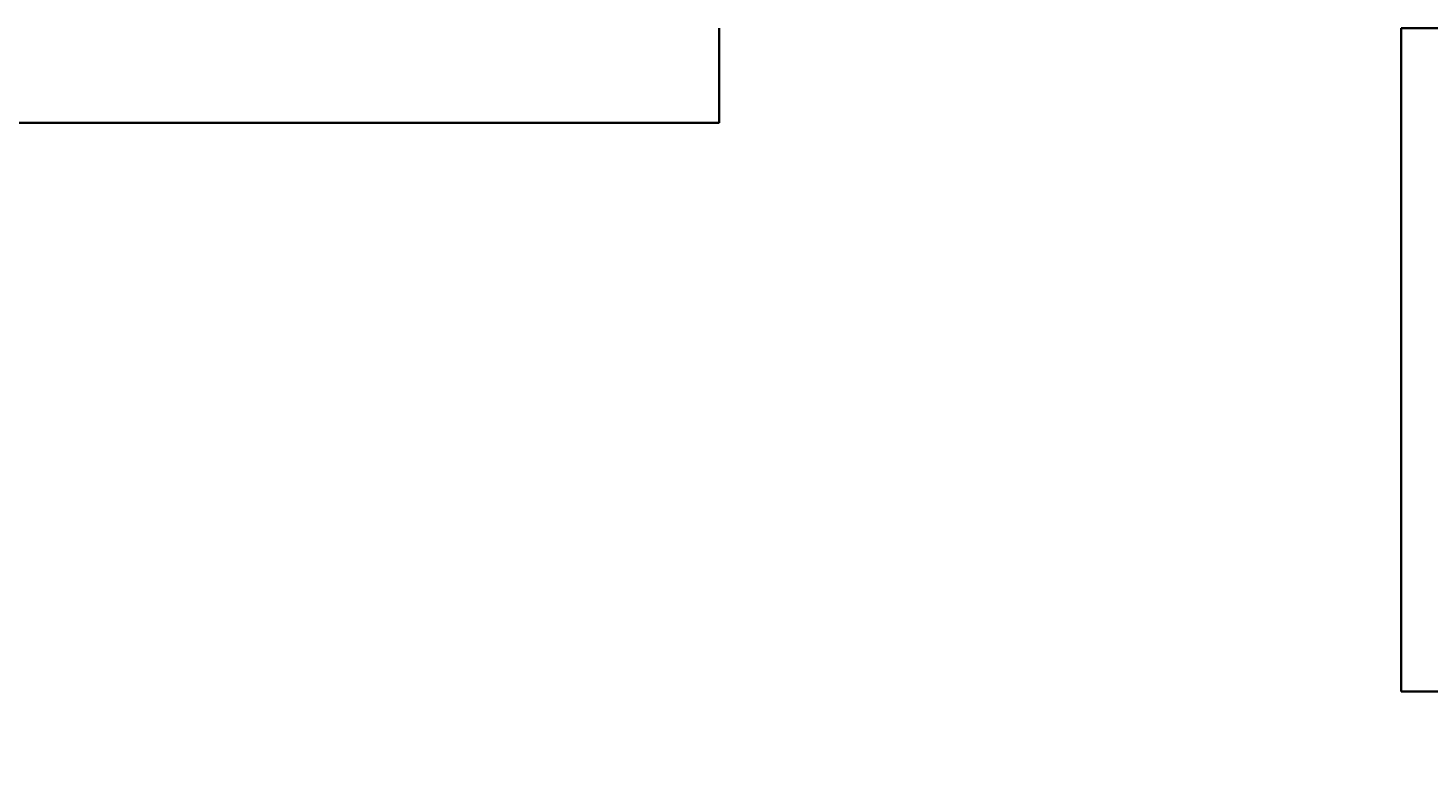
# Model space of a CAD drawing. Units: inches. Extents: x 3731 to 4318, y 1310 to 2388.
# Tile 7 of 57: x 3870 to 3944, y 1515 to 1554. Entities that reach past the tile are written whole.
import ezdxf

# ---------------------------------------------------------------- set-up
doc = ezdxf.new("R2010")
doc.units = ezdxf.units.IN
doc.layers.add('A-ANNO-DIMS', color=2, linetype='Continuous', lineweight=18)
doc.layers.add('A-WALL', color=7, linetype='Continuous', lineweight=35)
doc.styles.get("Standard").update_dxf_attribs({"font": 'arial.ttf'})
doc.dimstyles.get("Standard").update_dxf_attribs({"dimtxt": 0.18, "dimasz": 0.18, "dimexe": 0.18, "dimexo": 0.0625, "dimgap": 0.09, "dimtad": 0, "dimtih": 1, "dimtoh": 1, "dimdec": 4, "dimzin": 0, "dimdsep": 46, "dimtxsty": 'Standard', "dimcen": 0.09, "dimadec": 0, "dimazin": 0, "dimtfac": 1, "dimtdec": 4, "dimtofl": 0, "dimtmove": 0, "dimatfit": 3, "dimfxl": 1, "dimtolj": 1, "dimtzin": 0, "dimarcsym": 0})

# ---------------------------------------------------------------- blocks, each defined once
blk = doc.blocks.new('*D32')
at = {"layer": 'A-ANNO-DIMS', "color": 0, "lineweight": -2, "transparency": 16777216}
for p, q in [((4269.211, 1592.319), (4269.211, 1310.251)), ((3835.209, 1359.319), (3835.209, 1310.251)), ((3835.389, 1310.431), (4051.918, 1310.431)), ((4269.031, 1310.431), (4052.502, 1310.431))]:
    blk.add_line(p, q, dxfattribs=at)
at = {"layer": 'A-ANNO-DIMS', "color": 0, "transparency": 16777216}
for points in [[(3835.389, 1310.461), (3835.389, 1310.401), (3835.209, 1310.431)], [(4269.031, 1310.461), (4269.031, 1310.401), (4269.211, 1310.431)]]:
    blk.add_solid(points, dxfattribs=at)
at = {"layer": 'Defpoints', "color": 0, "transparency": 16777216}
for p in [(4269.211, 1592.382), (3835.209, 1359.382), (4269.211, 1310.431)]:
    blk.add_point(p, dxfattribs=at)
at = {"layer": 'A-ANNO-DIMS', "color": 0, "transparency": 16777216, "insert": (4052.21, 1310.431), "char_height": 0.18, "attachment_point": 5}
blk.add_mtext('\\A1;434', dxfattribs=at)

msp = doc.modelspace()

# ---------------------------------------------------------------- linework, layer by layer
at = {"layer": 'A-WALL'}
for p, q in [((3906.211, 1554.382), (3906.211, 1549.382)), ((3942.211, 1554.382), (3942.211, 1519.382)), ((3942.211, 1554.382), (4067.209, 1554.382)), ((3840.209, 1549.382), (3906.211, 1549.382)), ((3942.211, 1519.382), (3947.211, 1519.382))]:
    msp.add_line(p, q, dxfattribs=at)

# ---------------------------------------------------------------- dimensions: what is measured, and where the dimension line sits
at = {"layer": 'A-ANNO-DIMS'}
dim = msp.add_linear_dim(base=(4269.211, 1310.431), p1=(3835.209, 1359.382), p2=(4269.211, 1592.382), dimstyle='Standard', override={"dimdec": 0, "dimlfac": 1, "dimrnd": 0, "dimzin": 0, "dimdsep": 46, "dimlunit": 2}, dxfattribs=at)
dim.commit()
dim.dimension.update_dxf_attribs({"geometry": '*D32', "text_midpoint": (4052.21, 1310.431)})

doc.saveas('drawing.dxf')
